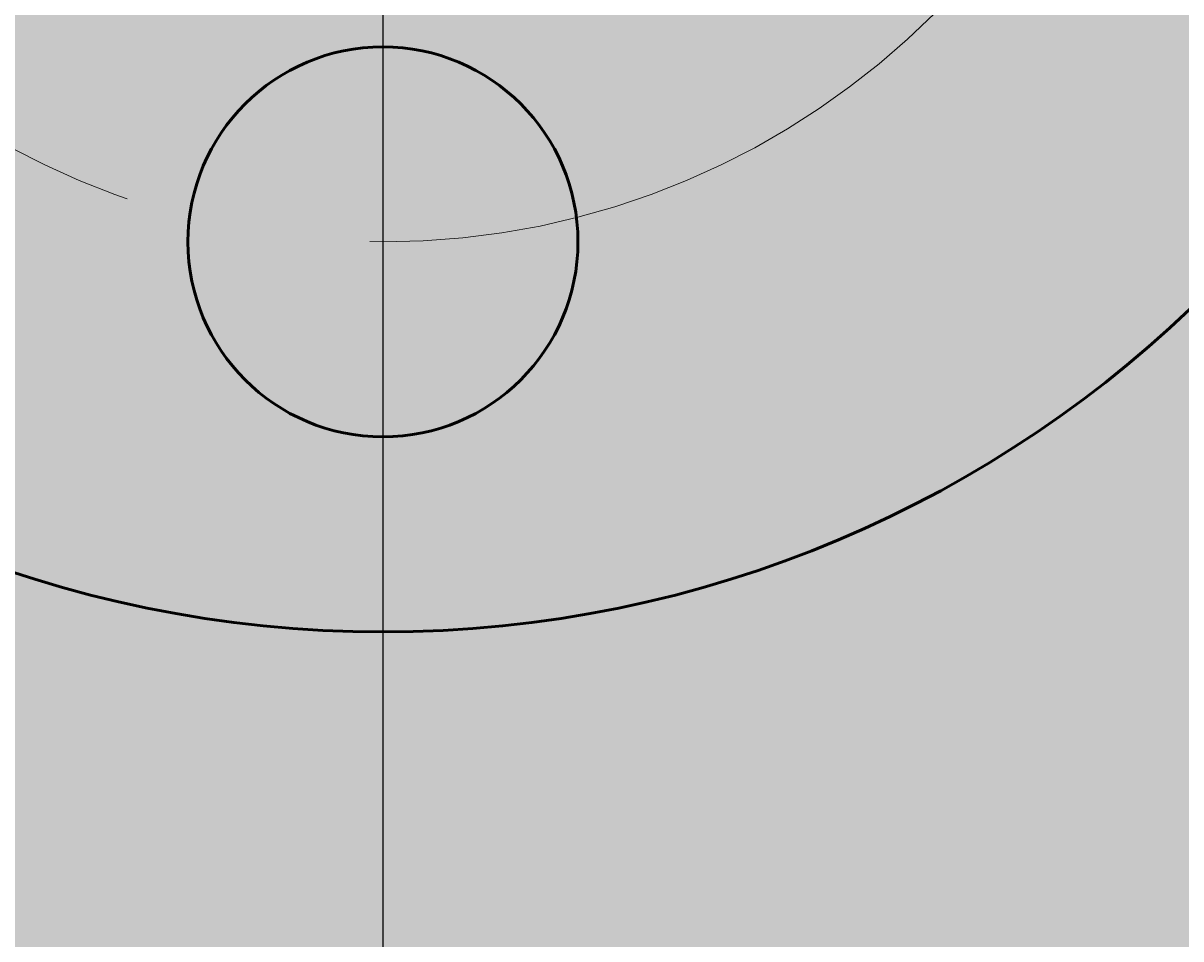
# Model space of a CAD drawing. Units: inches. Extents: x 114 to 236, y -51 to 115.
# Tile 9 of 14: x 166 to 196, y 41 to 65. Entities that reach past the tile are written whole.
import ezdxf

# ---------------------------------------------------------------- set-up
doc = ezdxf.new("R2010")
doc.units = ezdxf.units.IN
doc.header["$MEASUREMENT"] = 0
doc.linetypes.add('CENTER', pattern=[50.8, 31.75, -6.35, 6.35, -6.35])
for name, color, linetype, lineweight in [('M-CNTR', 7, 'CENTER', 18), ('M-DIMS', 2, 'Continuous', 18), ('M-OUTL', 7, 'Continuous', 50)]:
    doc.layers.add(name, color=color, linetype=linetype, lineweight=lineweight)
doc.layers.add('M-HATC', color=7, linetype='Continuous', lineweight=18, true_color=0xffffff)
doc.styles.get("Standard").update_dxf_attribs({"font": 'arial.ttf'})
doc.dimstyles.get("Standard").update_dxf_attribs({"dimtxt": 0.18, "dimasz": 0.18, "dimexe": 0.18, "dimexo": 0.0625, "dimgap": 0.09, "dimtad": 0, "dimtih": 1, "dimtoh": 1, "dimdec": 4, "dimzin": 0, "dimdsep": 46, "dimtxsty": 'Standard', "dimcen": 0.09, "dimadec": 0, "dimazin": 0, "dimtfac": 1, "dimtdec": 4, "dimtofl": 0, "dimtmove": 0, "dimatfit": 3, "dimfxl": 1, "dimtolj": 1, "dimtzin": 0, "dimarcsym": 0})

# ---------------------------------------------------------------- blocks, each defined once
blk = doc.blocks.new('BOLT-HOLE-D10')
blk.add_circle((0, 0), 5)
blk = doc.blocks.new('*D3')
at = {"layer": 'Defpoints', "color": 0, "transparency": 16777216}
for p in [(230.229, 115.287), (120.229, 9.307), (230.229, 9.307)]:
    blk.add_point(p, dxfattribs=at)
at = {"layer": 'M-DIMS', "color": 0, "lineweight": -2, "transparency": 16777216}
for p, q in [((120.229, 9.37), (120.229, 115.467)), ((230.229, 9.37), (230.229, 115.467)), ((120.409, 115.287), (174.949, 115.287)), ((230.049, 115.287), (175.509, 115.287))]:
    blk.add_line(p, q, dxfattribs=at)
at = {"layer": 'M-DIMS', "color": 0, "transparency": 16777216}
for points in [[(120.409, 115.317), (120.409, 115.257), (120.229, 115.287)], [(230.049, 115.317), (230.049, 115.257), (230.229, 115.287)]]:
    blk.add_solid(points, dxfattribs=at)
at = {"layer": 'M-DIMS', "color": 0, "transparency": 16777216, "insert": (175.229, 115.287), "char_height": 0.18, "attachment_point": 5}
blk.add_mtext('\\A1;110', dxfattribs=at)
blk = doc.blocks.new('*D4')
at = {"layer": 'Defpoints', "color": 0, "transparency": 16777216}
for p in [(114.249, 109.307), (175.229, 109.307), (135.229, -5.693)]:
    blk.add_point(p, dxfattribs=at)
at = {"layer": 'M-DIMS', "color": 0, "lineweight": -2, "transparency": 16777216}
for p, q in [((175.166, 109.307), (114.069, 109.307)), ((114.249, 109.127), (114.249, 51.989)), ((114.249, -5.513), (114.249, 51.625)), ((135.166, -5.693), (114.069, -5.693))]:
    blk.add_line(p, q, dxfattribs=at)
at = {"layer": 'M-DIMS', "color": 0, "transparency": 16777216}
for points in [[(114.219, 109.127), (114.279, 109.127), (114.249, 109.307)], [(114.219, -5.513), (114.279, -5.513), (114.249, -5.693)]]:
    blk.add_solid(points, dxfattribs=at)
at = {"layer": 'M-DIMS', "color": 0, "transparency": 16777216, "insert": (114.249, 51.807), "char_height": 0.18, "attachment_point": 5}
blk.add_mtext('\\A1;115', dxfattribs=at)
blk = doc.blocks.new('*D5')
at = {"layer": 'Defpoints', "color": 0, "transparency": 16777216}
for p in [(175.229, 79.307), (135.229, 9.307), (175.229, -11.673)]:
    blk.add_point(p, dxfattribs=at)
at = {"layer": 'M-DIMS', "color": 0, "lineweight": -2, "transparency": 16777216}
for p, q in [((175.229, 79.245), (175.229, -11.853)), ((135.229, 9.245), (135.229, -11.853)), ((135.409, -11.673), (155.006, -11.673)), ((175.049, -11.673), (155.451, -11.673))]:
    blk.add_line(p, q, dxfattribs=at)
at = {"layer": 'M-DIMS', "color": 0, "transparency": 16777216}
for points in [[(135.409, -11.643), (135.409, -11.703), (135.229, -11.673)], [(175.049, -11.643), (175.049, -11.703), (175.229, -11.673)]]:
    blk.add_solid(points, dxfattribs=at)
at = {"layer": 'M-DIMS', "color": 0, "transparency": 16777216, "insert": (155.229, -11.673), "char_height": 0.18, "attachment_point": 5}
blk.add_mtext('\\A1;40', dxfattribs=at)
blk = doc.blocks.new('*D6')
at = {"layer": 'Defpoints', "color": 0, "transparency": 16777216}
for p in [(175.229, 79.307), (215.229, 9.307), (215.229, -11.673)]:
    blk.add_point(p, dxfattribs=at)
at = {"layer": 'M-DIMS', "color": 0, "lineweight": -2, "transparency": 16777216}
for p, q in [((175.229, 79.245), (175.229, -11.853)), ((215.229, 9.245), (215.229, -11.853)), ((175.409, -11.673), (195.006, -11.673)), ((215.049, -11.673), (195.451, -11.673))]:
    blk.add_line(p, q, dxfattribs=at)
at = {"layer": 'M-DIMS', "color": 0, "transparency": 16777216}
for points in [[(175.409, -11.643), (175.409, -11.703), (175.229, -11.673)], [(215.049, -11.643), (215.049, -11.703), (215.229, -11.673)]]:
    blk.add_solid(points, dxfattribs=at)
at = {"layer": 'M-DIMS', "color": 0, "transparency": 16777216, "insert": (195.229, -11.673), "char_height": 0.18, "attachment_point": 5}
blk.add_mtext('\\A1;40', dxfattribs=at)
blk = doc.blocks.new('*D7')
at = {"layer": 'Defpoints', "color": 0, "transparency": 16777216}
for p in [(175.229, 79.307), (236.209, 79.307), (215.229, 9.307)]:
    blk.add_point(p, dxfattribs=at)
at = {"layer": 'M-DIMS', "color": 0, "lineweight": -2, "transparency": 16777216}
for p, q in [((175.291, 79.307), (236.389, 79.307)), ((236.209, 79.127), (236.209, 44.489)), ((236.209, 9.487), (236.209, 44.125)), ((215.291, 9.307), (236.389, 9.307))]:
    blk.add_line(p, q, dxfattribs=at)
at = {"layer": 'M-DIMS', "color": 0, "transparency": 16777216}
for points in [[(236.179, 79.127), (236.239, 79.127), (236.209, 79.307)], [(236.179, 9.487), (236.239, 9.487), (236.209, 9.307)]]:
    blk.add_solid(points, dxfattribs=at)
at = {"layer": 'M-DIMS', "color": 0, "transparency": 16777216, "insert": (236.209, 44.307), "char_height": 0.18, "attachment_point": 5}
blk.add_mtext('\\A1;70', dxfattribs=at)
blk = doc.blocks.new('*D8')
at = {"layer": 'Defpoints', "color": 0, "transparency": 16777216}
for p in [(197.149, 99.789), (153.308, 58.825)]:
    blk.add_point(p, dxfattribs=at)
at = {"layer": 'M-DIMS', "color": 0, "lineweight": -2, "transparency": 16777216}
for p, q in [((210.301, 112.078), (197.28, 99.912)), ((210.481, 112.078), (210.301, 112.078)), ((175.139, 79.307), (175.319, 79.307)), ((175.229, 79.217), (175.229, 79.397))]:
    blk.add_line(p, q, dxfattribs=at)
at = {"layer": 'M-DIMS', "color": 0, "transparency": 16777216}
blk.add_solid([(197.26, 99.934), (197.301, 99.89), (197.149, 99.789)], dxfattribs=at)
at = {"layer": 'M-DIMS', "color": 0, "transparency": 16777216, "insert": (210.797, 112.078), "char_height": 0.18, "attachment_point": 5}
blk.add_mtext('\\A1;∅60', dxfattribs=at)

msp = doc.modelspace()

# ---------------------------------------------------------------- hatches: boundary and pattern name
at = {"layer": 'M-HATC'}
h = msp.add_hatch(color=256, dxfattribs=at)
h.set_gradient(color1=(19, 155, 72), color2=(255, 255, 0), tint=1, name='HEMISPHERICAL')
h.paths.add_polyline_path([(147.853, 91.577), (146.105, 86.505, 0.060651), (145.229, 79.307, 1), (205.229, 79.307, 0.060651), (204.352, 86.505), (202.605, 91.577, 0.647643)])
h.paths.add_polyline_path([(180.229, 99.307, -0.031342), (180.189, 98.682, -0.27393), (194.604, 84.268, -0.451416), (200.229, 79.307, -0.451416), (194.604, 74.346, -0.27393), (180.189, 59.932, -0.031342), (180.229, 59.307, -1), (170.229, 59.307, -0.031342), (170.268, 59.932, -0.27393), (155.854, 74.346, -0.451416), (150.229, 79.307, -0.451416), (155.854, 84.268, -0.27393), (170.268, 98.682, -0.031342), (170.229, 99.307, -1)], flags=16)
h.paths.add_polyline_path([(183.229, 79.307, -1), (167.229, 79.307, -1)], flags=0)
h.paths.add_polyline_path([(155.854, 84.268, -0.377964), (160.229, 79.307, -0.377964), (155.854, 74.346, 0.27393), (170.268, 59.932, -0.881917), (180.189, 59.932, 0.27393), (194.604, 74.346, -0.377964), (190.229, 79.307, -0.377964), (194.604, 84.268, 0.27393), (180.189, 98.682, -0.881917), (170.268, 98.682, 0.27393)], flags=0)
h = msp.add_hatch(color=256, dxfattribs=at)
h.set_gradient(color1=(242, 103, 34), color2=(255, 255, 0), tint=1, name='INVSPHERICAL')
h.paths.add_polyline_path([(145.229, 79.307, -0.060651), (146.105, 86.505), (121.823, 16.038, -0.790743), (150.229, 9.307, -0.236068), (144.229, -2.693, -0.14094), (175.229, 9.098, -0.14094), (206.229, -2.693, -0.236068), (200.229, 9.307, -0.790743), (228.634, 16.038), (204.352, 86.505, -0.060651), (205.229, 79.307, -1)])
h = msp.add_hatch(color=256, dxfattribs=at)
h.paths.add_polyline_path([(180.229, 59.307, 0.031342), (180.189, 59.932, -0.125988), (170.268, 59.932, 0.031342), (170.229, 59.307, 1)])
h.paths.add_polyline_path([(170.268, 59.932, 0.125988), (180.189, 59.932, 0.881917)])

# ---------------------------------------------------------------- linework, layer by layer
at = {"layer": 'M-CNTR'}
msp.add_circle((175.229, 79.307), 20, dxfattribs=at)
at = {"layer": 'M-OUTL'}
msp.add_circle((175.229, 79.307), 30, dxfattribs=at)

# ---------------------------------------------------------------- block references
msp.add_blockref('BOLT-HOLE-D10', (175.229, 59.307), dxfattribs=at)

# ---------------------------------------------------------------- dimensions: what is measured, and where the dimension line sits
at = {"layer": 'M-DIMS'}
for base, p1, p2, picture, middle in [((230.229, 115.287), (120.229, 9.307), (230.229, 9.307), '*D3', (175.229, 115.287)), ((175.229, -11.673), (135.229, 9.307), (175.229, 79.307), '*D5', (155.229, -11.673)), ((215.229, -11.673), (175.229, 79.307), (215.229, 9.307), '*D6', (195.229, -11.673))]:
    dim = msp.add_linear_dim(base=base, p1=p1, p2=p2, dimstyle='Standard', override={"dimdec": 0, "dimlfac": 1, "dimrnd": 0, "dimzin": 0, "dimdsep": 46, "dimlunit": 2}, dxfattribs=at)
    dim.commit()
    dim.dimension.update_dxf_attribs({"geometry": picture, "text_midpoint": middle})
dim = msp.add_diameter_dim_2p(p1=(153.308, 58.825), p2=(197.149, 99.789), dimstyle='Standard', override={"dimdec": 0, "dimlfac": 1, "dimrnd": 0, "dimzin": 0, "dimdsep": 46, "dimlunit": 2}, dxfattribs=at)
dim.commit()
dim.dimension.update_dxf_attribs({"geometry": '*D8', "text_midpoint": (210.797, 112.078), "dimtype": 163})
for base, p1, p2, picture, middle in [((114.249, 109.307), (135.229, -5.693), (175.229, 109.307), '*D4', (114.249, 51.807)), ((236.209, 79.307), (215.229, 9.307), (175.229, 79.307), '*D7', (236.209, 44.307))]:
    dim = msp.add_linear_dim(base=base, p1=p1, p2=p2, angle=90, dimstyle='Standard', override={"dimdec": 0, "dimlfac": 1, "dimrnd": 0, "dimzin": 0, "dimdsep": 46, "dimlunit": 2}, dxfattribs=at)
    dim.commit()
    dim.dimension.update_dxf_attribs({"geometry": picture, "text_midpoint": middle})

doc.saveas('drawing.dxf')
